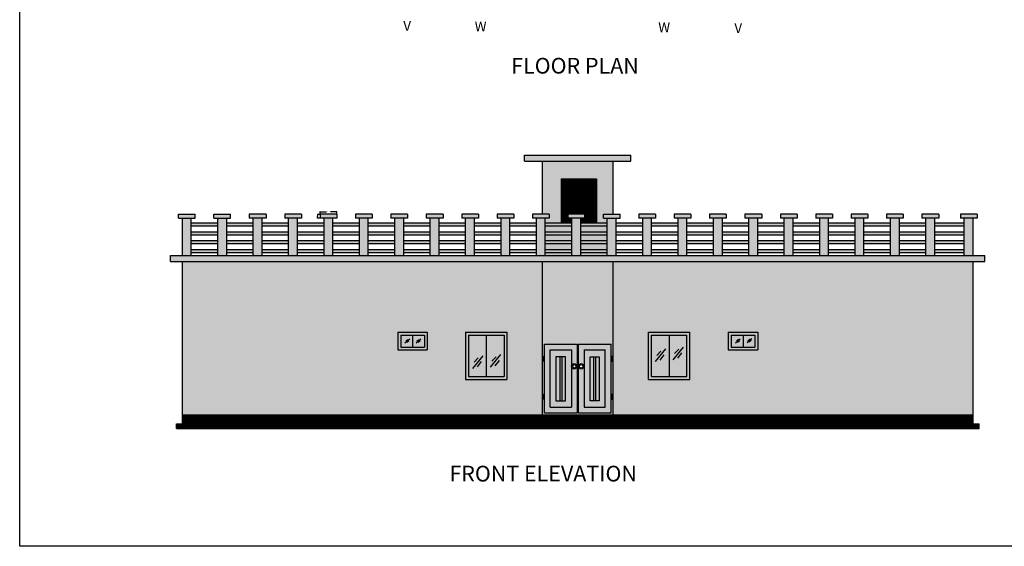
# Model space of a CAD drawing. Units: inches. Extents: x 9239 to 26065, y 6728 to 14611.
# Tile 1 of 12: x 9239 to 10240, y 6728 to 7264. Entities that reach past the tile are written whole.
import ezdxf

# ---------------------------------------------------------------- set-up
doc = ezdxf.new("R2010")
doc.units = ezdxf.units.IN
doc.header["$MEASUREMENT"] = 0
for name, color, linetype, lineweight in [('A-ANNO-DIMS', 2, 'Continuous', 18), ('A-ANNO-TEXT', 7, 'Continuous', 18), ('A-ELEV', 7, 'Continuous', 25), ('A-ELEV-PATT', 252, 'Continuous', 13), ('A-FLOR-STRS', 3, 'Continuous', 25)]:
    doc.layers.add(name, color=color, linetype=linetype, lineweight=lineweight)
doc.styles.get("Standard").update_dxf_attribs({"font": 'arial.ttf'})
doc.dimstyles.get("Standard").update_dxf_attribs({"dimtxt": 0.18, "dimasz": 0.18, "dimexe": 0.18, "dimexo": 0.0625, "dimgap": 0.09, "dimtad": 0, "dimtih": 1, "dimtoh": 1, "dimdec": 0, "dimzin": 0, "dimdsep": 46, "dimlunit": 3, "dimtxsty": 'Standard', "dimcen": 0.09, "dimadec": 0, "dimazin": 0, "dimtfac": 1, "dimtdec": 0, "dimtofl": 0, "dimtmove": 0, "dimatfit": 3, "dimfxl": 1, "dimtolj": 1, "dimtzin": 0, "dimarcsym": 0})

# ---------------------------------------------------------------- blocks, each defined once
blk = doc.blocks.new('ELEV-RAIL-POST')
for p, q in [((0, 4), (17, 4)), ((0, 0), (0, 4)), ((17, 0), (17, 4)), ((0, 0), (17, 0))]:
    blk.add_line(p, q)
blk = doc.blocks.new('*D48')
at = {"layer": 'A-ANNO-DIMS', "color": 0, "lineweight": -2, "transparency": 16777216}
for p, q in [((9544, 7065.9), (9544, 7068.6)), ((9544.2, 7068.4), (9550.6, 7068.4)), ((9560.9, 7068.4), (9554.5, 7068.4)), ((9561, 7065.9), (9561, 7068.6))]:
    blk.add_line(p, q, dxfattribs=at)
at = {"layer": 'A-ANNO-DIMS', "color": 0, "transparency": 16777216}
for points in [[(9544.2, 7068.4), (9544.2, 7068.4), (9544, 7068.4)], [(9560.9, 7068.4), (9560.9, 7068.4), (9561, 7068.4)]]:
    blk.add_solid(points, dxfattribs=at)
at = {"layer": 'Defpoints', "color": 0, "transparency": 16777216}
for p in [(9544, 7068.4), (9544, 7065.8), (9561, 7065.8)]:
    blk.add_point(p, dxfattribs=at)
at = {"layer": 'A-ANNO-DIMS', "color": 0, "transparency": 16777216, "insert": (9552.5, 7068.4), "char_height": 0.18, "attachment_point": 5}
blk.add_mtext('\\A1;PARAPET RAIL POST 1\'-5" TYP.', dxfattribs=at)
blk = doc.blocks.new('*D49')
at = {"layer": 'A-ANNO-DIMS', "color": 0, "lineweight": -2, "transparency": 16777216}
for p, q in [((9544, 7065.8), (9541.3, 7065.8)), ((9544, 7061.8), (9541.3, 7061.8)), ((9541.5, 7065.7), (9541.5, 7064)), ((9541.5, 7062), (9541.5, 7063.7))]:
    blk.add_line(p, q, dxfattribs=at)
at = {"layer": 'A-ANNO-DIMS', "color": 0, "transparency": 16777216}
for points in [[(9541.5, 7065.7), (9541.5, 7065.7), (9541.5, 7065.8)], [(9541.5, 7062), (9541.5, 7062), (9541.5, 7061.8)]]:
    blk.add_solid(points, dxfattribs=at)
at = {"layer": 'Defpoints', "color": 0, "transparency": 16777216}
for p in [(9541.5, 7061.8), (9544, 7065.8), (9544, 7061.8)]:
    blk.add_point(p, dxfattribs=at)
at = {"layer": 'A-ANNO-DIMS', "color": 0, "transparency": 16777216, "insert": (9541.5, 7063.8), "char_height": 0.18, "attachment_point": 5}
blk.add_mtext('\\A1;0\'-4" TYP.', dxfattribs=at)

msp = doc.modelspace()

# ---------------------------------------------------------------- hatches: boundary and pattern name
at = {"layer": 'A-ELEV-PATT'}
h = msp.add_hatch(color=256, dxfattribs=at)
h.dxf.hatch_style = 1
h.paths.add_polyline_path([(9752.05, 7125.85), (9752.05, 7119.85), (9860.05, 7119.85), (9860.05, 7125.85)])
h = msp.add_hatch(color=256, dxfattribs=at)
h.dxf.hatch_style = 1
h.paths.add_polyline_path([(9770.05, 7065.85), (9777.05, 7065.85), (9777.05, 7061.85), (9773.05, 7061.85), (9773.05, 7057.11), (9789.16, 7057.11), (9789.16, 7101.85), (9825.16, 7101.85), (9825.16, 7057.11), (9836.05, 7057.11), (9836.05, 7061.85), (9832.05, 7061.85), (9832.05, 7065.85), (9842.05, 7065.85), (9842.05, 7119.85), (9770.05, 7119.85)])
h.paths.add_polyline_path([(9800.05, 7048.11), (9800.05, 7054.11), (9773.05, 7054.11), (9773.05, 7048.11)])
h.paths.add_polyline_path([(9773.05, 7045.11), (9773.05, 7039.11), (9800.05, 7039.11), (9800.05, 7045.11)])
h.paths.add_polyline_path([(9773.05, 7036.11), (9773.05, 7030.11), (9800.05, 7030.11), (9800.05, 7036.11)])
h.paths.add_polyline_path([(9773.05, 7027.11), (9773.05, 7023.85), (9800.05, 7023.85), (9800.05, 7027.11)])
h.paths.add_polyline_path([(9836.05, 7023.85), (9836.05, 7027.11), (9809.05, 7027.11), (9809.05, 7023.85)])
h.paths.add_polyline_path([(9809.05, 7036.11), (9809.05, 7030.11), (9836.05, 7030.11), (9836.05, 7036.11)])
h.paths.add_polyline_path([(9809.05, 7045.11), (9809.05, 7039.11), (9836.05, 7039.11), (9836.05, 7045.11)])
h.paths.add_polyline_path([(9809.05, 7054.11), (9809.05, 7048.11), (9836.05, 7048.11), (9836.05, 7054.11)])
h = msp.add_hatch(dxfattribs=at)
h.set_pattern_fill('ANSI31', color=256)
h.set_pattern_definition([(45, (9789.16169, 7057.11151), (-0.08838835, 0.08838835), [])])
h.paths.add_polyline_path([(9825.16, 7101.85), (9789.16, 7101.85), (9789.16, 7057.11), (9794.16, 7057.11), (9794.16, 7096.85), (9820.16, 7096.85), (9820.16, 7057.11), (9825.16, 7057.11)])
h.paths.add_polyline_path([(9814.34, 7090.65), (9799.4, 7090.65), (9799.4, 7065.85), (9813.05, 7065.85), (9813.05, 7061.85), (9809.05, 7061.85), (9809.05, 7057.11), (9814.34, 7057.11)], flags=17)
h = msp.add_hatch(dxfattribs=at)
h.set_pattern_fill('ANSI31', color=256)
h.set_pattern_definition([(45, (9794.16169, 7057.11151), (-0.08838835, 0.08838835), [])])
h.paths.add_polyline_path([(9799.4, 7090.65), (9814.34, 7090.65), (9814.34, 7057.11), (9820.16, 7057.11), (9820.16, 7096.85), (9794.16, 7096.85), (9794.16, 7057.11), (9800.05, 7057.11), (9800.05, 7061.85), (9796.05, 7061.85), (9796.05, 7065.85), (9799.4, 7065.85)])
h = msp.add_hatch(color=256, dxfattribs=at)
h.dxf.hatch_style = 1
h.paths.add_polyline_path([(9392.05, 7023.85), (9392.05, 7017.85), (10220.05, 7017.85), (10220.05, 7023.85)])
h.paths.add_polyline_path([(9400.05, 7065.85), (9400.05, 7061.85), (9417.05, 7061.85), (9417.05, 7065.85)])
h.paths.add_polyline_path([(9453.05, 7061.85), (9453.05, 7065.85), (9436.05, 7065.85), (9436.05, 7061.85)])
h.paths.add_polyline_path([(9489.05, 7061.85), (9489.05, 7065.85), (9472.05, 7065.85), (9472.05, 7061.85)])
h.paths.add_polyline_path([(9525.05, 7065.85), (9508.05, 7065.85), (9508.05, 7061.85), (9525.05, 7061.85)])
h.paths.add_polyline_path([(9544.05, 7065.85), (9544.05, 7061.85), (9561.05, 7061.85), (9561.05, 7065.85)])
h.paths.add_polyline_path([(9597.05, 7061.85), (9597.05, 7065.85), (9580.05, 7065.85), (9580.05, 7061.85)])
h.paths.add_polyline_path([(9616.05, 7065.85), (9616.05, 7061.85), (9633.05, 7061.85), (9633.05, 7065.85)])
h.paths.add_polyline_path([(9652.05, 7065.85), (9652.05, 7061.85), (9669.05, 7061.85), (9669.05, 7065.85)])
h.paths.add_polyline_path([(9688.05, 7065.85), (9688.05, 7061.85), (9705.05, 7061.85), (9705.05, 7065.85)])
h.paths.add_polyline_path([(9741.05, 7061.85), (9741.05, 7065.85), (9724.05, 7065.85), (9724.05, 7061.85)])
h.paths.add_polyline_path([(9760.05, 7065.85), (9760.05, 7061.85), (9777.05, 7061.85), (9777.05, 7065.85)])
h.paths.add_polyline_path([(9796.05, 7065.85), (9796.05, 7061.85), (9813.05, 7061.85), (9813.05, 7065.85)])
h.paths.add_polyline_path([(9842.05, 7061.85), (9849.05, 7061.85), (9849.05, 7065.85), (9842.05, 7065.85), (9832.05, 7065.85), (9832.05, 7061.85)])
h.paths.add_polyline_path([(9885.05, 7061.85), (9885.05, 7065.85), (9868.05, 7065.85), (9868.05, 7061.85)])
h.paths.add_polyline_path([(9921.05, 7061.85), (9921.05, 7065.85), (9904.05, 7065.85), (9904.05, 7061.85)])
h.paths.add_polyline_path([(9940.05, 7065.85), (9940.05, 7061.85), (9957.05, 7061.85), (9957.05, 7065.85)])
h.paths.add_polyline_path([(9976.05, 7065.85), (9976.05, 7061.85), (9993.05, 7061.85), (9993.05, 7065.85)])
h.paths.add_polyline_path([(10029.05, 7065.85), (10012.05, 7065.85), (10012.05, 7061.85), (10029.05, 7061.85)])
h.paths.add_polyline_path([(10048.05, 7065.85), (10048.05, 7061.85), (10065.05, 7061.85), (10065.05, 7065.85)])
h.paths.add_polyline_path([(10101.05, 7061.85), (10101.05, 7065.85), (10084.05, 7065.85), (10084.05, 7061.85)])
h.paths.add_polyline_path([(10173.05, 7061.85), (10173.05, 7065.85), (10156.05, 7065.85), (10156.05, 7061.85)])
h.paths.add_polyline_path([(10137.05, 7061.85), (10137.05, 7065.85), (10120.05, 7065.85), (10120.05, 7061.85)])
h.paths.add_polyline_path([(10212.05, 7061.85), (10212.05, 7065.85), (10195.05, 7065.85), (10195.05, 7061.85)])
h = msp.add_hatch(color=256, dxfattribs=at)
h.dxf.hatch_style = 1
h.paths.add_polyline_path([(9404.05, 7023.85), (9413.05, 7023.85), (9413.05, 7061.85), (9404.05, 7061.85)])
h.paths.add_polyline_path([(9449.05, 7061.85), (9440.05, 7061.85), (9440.05, 7023.85), (9449.05, 7023.85)])
h.paths.add_polyline_path([(9476.05, 7023.85), (9485.05, 7023.85), (9485.05, 7061.85), (9476.05, 7061.85)])
h.paths.add_polyline_path([(9521.05, 7061.85), (9512.05, 7061.85), (9512.05, 7023.85), (9521.05, 7023.85)])
h.paths.add_polyline_path([(9557.05, 7061.85), (9548.05, 7061.85), (9548.05, 7023.85), (9557.05, 7023.85)])
h.paths.add_polyline_path([(9584.05, 7023.85), (9593.05, 7023.85), (9593.05, 7061.85), (9584.05, 7061.85)])
h.paths.add_polyline_path([(9620.05, 7023.85), (9629.05, 7023.85), (9629.05, 7061.85), (9620.05, 7061.85)])
h.paths.add_polyline_path([(9665.05, 7061.85), (9656.05, 7061.85), (9656.05, 7023.85), (9665.05, 7023.85)])
h.paths.add_polyline_path([(9692.05, 7023.85), (9701.05, 7023.85), (9701.05, 7061.85), (9692.05, 7061.85)])
h.paths.add_polyline_path([(9728.05, 7023.85), (9737.05, 7023.85), (9737.05, 7061.85), (9728.05, 7061.85)])
h.paths.add_polyline_path([(9773.05, 7061.85), (9764.05, 7061.85), (9764.05, 7023.85), (9773.05, 7023.85)])
h.paths.add_polyline_path([(9809.05, 7061.85), (9800.05, 7061.85), (9800.05, 7023.85), (9809.05, 7023.85)])
h.paths.add_polyline_path([(9845.05, 7061.85), (9842.05, 7061.85), (9836.05, 7061.85), (9836.05, 7023.85), (9845.05, 7023.85)])
h.paths.add_polyline_path([(9872.05, 7023.85), (9881.05, 7023.85), (9881.05, 7061.85), (9872.05, 7061.85)])
h.paths.add_polyline_path([(9917.05, 7061.85), (9908.05, 7061.85), (9908.05, 7023.85), (9917.05, 7023.85)])
h.paths.add_polyline_path([(9953.05, 7061.85), (9944.05, 7061.85), (9944.05, 7023.85), (9953.05, 7023.85)])
h.paths.add_polyline_path([(9980.05, 7023.85), (9989.05, 7023.85), (9989.05, 7061.85), (9980.05, 7061.85)])
h.paths.add_polyline_path([(10025.05, 7061.85), (10016.05, 7061.85), (10016.05, 7023.85), (10025.05, 7023.85)])
h.paths.add_polyline_path([(10061.05, 7061.85), (10052.05, 7061.85), (10052.05, 7023.85), (10061.05, 7023.85)])
h.paths.add_polyline_path([(10088.05, 7023.85), (10097.05, 7023.85), (10097.05, 7061.85), (10088.05, 7061.85)])
h.paths.add_polyline_path([(10133.05, 7061.85), (10124.05, 7061.85), (10124.05, 7023.85), (10133.05, 7023.85)])
h.paths.add_polyline_path([(10160.05, 7023.85), (10169.05, 7023.85), (10169.05, 7061.85), (10160.05, 7061.85)])
h.paths.add_polyline_path([(10208.05, 7061.85), (10199.05, 7061.85), (10199.05, 7023.85), (10208.05, 7023.85)])
h = msp.add_hatch(color=256, dxfattribs=at)
h.dxf.hatch_style = 1
h.paths.add_polyline_path([(9440.05, 7057.11), (9413.05, 7057.11), (9413.05, 7054.11), (9440.05, 7054.11)])
h.paths.add_polyline_path([(9440.05, 7048.11), (9413.05, 7048.11), (9413.05, 7045.11), (9440.05, 7045.11)])
h.paths.add_polyline_path([(9440.05, 7039.11), (9413.05, 7039.11), (9413.05, 7036.11), (9440.05, 7036.11)])
h.paths.add_polyline_path([(9440.05, 7030.11), (9413.05, 7030.11), (9413.05, 7027.11), (9440.05, 7027.11)])
h.paths.add_polyline_path([(9476.05, 7057.11), (9449.05, 7057.11), (9449.05, 7054.11), (9476.05, 7054.11)])
h.paths.add_polyline_path([(9476.05, 7048.11), (9449.05, 7048.11), (9449.05, 7045.11), (9476.05, 7045.11)])
h.paths.add_polyline_path([(9476.05, 7039.11), (9449.05, 7039.11), (9449.05, 7036.11), (9476.05, 7036.11)])
h.paths.add_polyline_path([(9476.05, 7030.11), (9449.05, 7030.11), (9449.05, 7027.11), (9476.05, 7027.11)])
h.paths.add_polyline_path([(9512.05, 7057.11), (9485.05, 7057.11), (9485.05, 7054.11), (9512.05, 7054.11)])
h.paths.add_polyline_path([(9512.05, 7048.11), (9485.05, 7048.11), (9485.05, 7045.11), (9512.05, 7045.11)])
h.paths.add_polyline_path([(9512.05, 7039.11), (9485.05, 7039.11), (9485.05, 7036.11), (9512.05, 7036.11)])
h.paths.add_polyline_path([(9512.05, 7030.11), (9485.05, 7030.11), (9485.05, 7027.11), (9512.05, 7027.11)])
h.paths.add_polyline_path([(9548.05, 7030.11), (9521.05, 7030.11), (9521.05, 7027.11), (9548.05, 7027.11)])
h.paths.add_polyline_path([(9548.05, 7039.11), (9521.05, 7039.11), (9521.05, 7036.11), (9548.05, 7036.11)])
h.paths.add_polyline_path([(9548.05, 7048.11), (9521.05, 7048.11), (9521.05, 7045.11), (9548.05, 7045.11)])
h.paths.add_polyline_path([(9548.05, 7057.11), (9521.05, 7057.11), (9521.05, 7054.11), (9548.05, 7054.11)])
h.paths.add_polyline_path([(9584.05, 7057.11), (9557.05, 7057.11), (9557.05, 7054.11), (9584.05, 7054.11)])
h.paths.add_polyline_path([(9620.05, 7057.11), (9593.05, 7057.11), (9593.05, 7054.11), (9620.05, 7054.11)])
h.paths.add_polyline_path([(9656.05, 7057.11), (9629.05, 7057.11), (9629.05, 7054.11), (9656.05, 7054.11)])
h.paths.add_polyline_path([(9656.05, 7048.11), (9629.05, 7048.11), (9629.05, 7045.11), (9656.05, 7045.11)])
h.paths.add_polyline_path([(9620.05, 7048.11), (9593.05, 7048.11), (9593.05, 7045.11), (9620.05, 7045.11)])
h.paths.add_polyline_path([(9584.05, 7048.11), (9557.05, 7048.11), (9557.05, 7045.11), (9584.05, 7045.11)])
h.paths.add_polyline_path([(9584.05, 7039.11), (9557.05, 7039.11), (9557.05, 7036.11), (9584.05, 7036.11)])
h.paths.add_polyline_path([(9620.05, 7039.11), (9593.05, 7039.11), (9593.05, 7036.11), (9620.05, 7036.11)])
h.paths.add_polyline_path([(9656.05, 7039.11), (9629.05, 7039.11), (9629.05, 7036.11), (9656.05, 7036.11)])
h.paths.add_polyline_path([(9656.05, 7030.11), (9629.05, 7030.11), (9629.05, 7027.11), (9656.05, 7027.11)])
h.paths.add_polyline_path([(9620.05, 7030.11), (9593.05, 7030.11), (9593.05, 7027.11), (9620.05, 7027.11)])
h.paths.add_polyline_path([(9584.05, 7030.11), (9557.05, 7030.11), (9557.05, 7027.11), (9584.05, 7027.11)])
h.paths.add_polyline_path([(9692.05, 7057.11), (9665.05, 7057.11), (9665.05, 7054.11), (9692.05, 7054.11)])
h.paths.add_polyline_path([(9728.05, 7057.11), (9701.05, 7057.11), (9701.05, 7054.11), (9728.05, 7054.11)])
h.paths.add_polyline_path([(9764.05, 7057.11), (9737.05, 7057.11), (9737.05, 7054.11), (9764.05, 7054.11)])
h.paths.add_polyline_path([(9764.05, 7048.11), (9737.05, 7048.11), (9737.05, 7045.11), (9764.05, 7045.11)])
h.paths.add_polyline_path([(9728.05, 7048.11), (9701.05, 7048.11), (9701.05, 7045.11), (9728.05, 7045.11)])
h.paths.add_polyline_path([(9692.05, 7048.11), (9665.05, 7048.11), (9665.05, 7045.11), (9692.05, 7045.11)])
h.paths.add_polyline_path([(9692.05, 7039.11), (9665.05, 7039.11), (9665.05, 7036.11), (9692.05, 7036.11)])
h.paths.add_polyline_path([(9728.05, 7039.11), (9701.05, 7039.11), (9701.05, 7036.11), (9728.05, 7036.11)])
h.paths.add_polyline_path([(9764.05, 7039.11), (9737.05, 7039.11), (9737.05, 7036.11), (9764.05, 7036.11)])
h.paths.add_polyline_path([(9692.05, 7030.11), (9665.05, 7030.11), (9665.05, 7027.11), (9692.05, 7027.11)])
h.paths.add_polyline_path([(9728.05, 7030.11), (9701.05, 7030.11), (9701.05, 7027.11), (9728.05, 7027.11)])
h.paths.add_polyline_path([(9764.05, 7030.11), (9737.05, 7030.11), (9737.05, 7027.11), (9764.05, 7027.11)])
h.paths.add_polyline_path([(9800.05, 7048.11), (9773.05, 7048.11), (9773.05, 7045.11), (9800.05, 7045.11)])
h.paths.add_polyline_path([(9800.05, 7057.11), (9773.05, 7057.11), (9773.05, 7054.11), (9800.05, 7054.11)])
h.paths.add_polyline_path([(9836.05, 7057.11), (9809.05, 7057.11), (9809.05, 7054.11), (9836.05, 7054.11)])
h.paths.add_polyline_path([(9836.05, 7048.11), (9809.05, 7048.11), (9809.05, 7045.11), (9836.05, 7045.11)])
h.paths.add_polyline_path([(9836.05, 7039.11), (9809.05, 7039.11), (9809.05, 7036.11), (9836.05, 7036.11)])
h.paths.add_polyline_path([(9800.05, 7039.11), (9773.05, 7039.11), (9773.05, 7036.11), (9800.05, 7036.11)])
h.paths.add_polyline_path([(9800.05, 7030.11), (9773.05, 7030.11), (9773.05, 7027.11), (9800.05, 7027.11)])
h.paths.add_polyline_path([(9836.05, 7030.11), (9809.05, 7030.11), (9809.05, 7027.11), (9836.05, 7027.11)])
h.paths.add_polyline_path([(9872.05, 7030.11), (9845.05, 7030.11), (9845.05, 7027.11), (9872.05, 7027.11)])
h.paths.add_polyline_path([(9872.05, 7039.11), (9845.05, 7039.11), (9845.05, 7036.11), (9872.05, 7036.11)])
h.paths.add_polyline_path([(9872.05, 7048.11), (9845.05, 7048.11), (9845.05, 7045.11), (9872.05, 7045.11)])
h.paths.add_polyline_path([(9872.05, 7057.11), (9845.05, 7057.11), (9845.05, 7054.11), (9872.05, 7054.11)])
h.paths.add_polyline_path([(9908.05, 7057.11), (9881.05, 7057.11), (9881.05, 7054.11), (9908.05, 7054.11)])
h.paths.add_polyline_path([(9908.05, 7048.11), (9881.05, 7048.11), (9881.05, 7045.11), (9908.05, 7045.11)])
h.paths.add_polyline_path([(9908.05, 7039.11), (9881.05, 7039.11), (9881.05, 7036.11), (9908.05, 7036.11)])
h.paths.add_polyline_path([(9908.05, 7030.11), (9881.05, 7030.11), (9881.05, 7027.11), (9908.05, 7027.11)])
h.paths.add_polyline_path([(9944.05, 7030.11), (9917.05, 7030.11), (9917.05, 7027.11), (9944.05, 7027.11)])
h.paths.add_polyline_path([(9944.05, 7039.11), (9917.05, 7039.11), (9917.05, 7036.11), (9944.05, 7036.11)])
h.paths.add_polyline_path([(9944.05, 7048.11), (9917.05, 7048.11), (9917.05, 7045.11), (9944.05, 7045.11)])
h.paths.add_polyline_path([(9944.05, 7057.11), (9917.05, 7057.11), (9917.05, 7054.11), (9944.05, 7054.11)])
h.paths.add_polyline_path([(9980.05, 7057.11), (9953.05, 7057.11), (9953.05, 7054.11), (9980.05, 7054.11)])
h.paths.add_polyline_path([(9980.05, 7048.11), (9953.05, 7048.11), (9953.05, 7045.11), (9980.05, 7045.11)])
h.paths.add_polyline_path([(9980.05, 7039.11), (9953.05, 7039.11), (9953.05, 7036.11), (9980.05, 7036.11)])
h.paths.add_polyline_path([(9980.05, 7030.11), (9953.05, 7030.11), (9953.05, 7027.11), (9980.05, 7027.11)])
h.paths.add_polyline_path([(10016.05, 7057.11), (9989.05, 7057.11), (9989.05, 7054.11), (10016.05, 7054.11)])
h.paths.add_polyline_path([(10016.05, 7048.11), (9989.05, 7048.11), (9989.05, 7045.11), (10016.05, 7045.11)])
h.paths.add_polyline_path([(10016.05, 7039.11), (9989.05, 7039.11), (9989.05, 7036.11), (10016.05, 7036.11)])
h.paths.add_polyline_path([(10052.05, 7057.11), (10025.05, 7057.11), (10025.05, 7054.11), (10052.05, 7054.11)])
h.paths.add_polyline_path([(10052.05, 7048.11), (10025.05, 7048.11), (10025.05, 7045.11), (10052.05, 7045.11)])
h.paths.add_polyline_path([(10052.05, 7039.11), (10025.05, 7039.11), (10025.05, 7036.11), (10052.05, 7036.11)])
h.paths.add_polyline_path([(10016.05, 7030.11), (9989.05, 7030.11), (9989.05, 7027.11), (10016.05, 7027.11)])
h.paths.add_polyline_path([(10052.05, 7030.11), (10025.05, 7030.11), (10025.05, 7027.11), (10052.05, 7027.11)])
h.paths.add_polyline_path([(10088.05, 7057.11), (10061.05, 7057.11), (10061.05, 7054.11), (10088.05, 7054.11)])
h.paths.add_polyline_path([(10088.05, 7048.11), (10061.05, 7048.11), (10061.05, 7045.11), (10088.05, 7045.11)])
h.paths.add_polyline_path([(10088.05, 7039.11), (10061.05, 7039.11), (10061.05, 7036.11), (10088.05, 7036.11)])
h.paths.add_polyline_path([(10088.05, 7030.11), (10061.05, 7030.11), (10061.05, 7027.11), (10088.05, 7027.11)])
h.paths.add_polyline_path([(10124.05, 7030.11), (10097.05, 7030.11), (10097.05, 7027.11), (10124.05, 7027.11)])
h.paths.add_polyline_path([(10124.05, 7039.11), (10097.05, 7039.11), (10097.05, 7036.11), (10124.05, 7036.11)])
h.paths.add_polyline_path([(10124.05, 7048.11), (10097.05, 7048.11), (10097.05, 7045.11), (10124.05, 7045.11)])
h.paths.add_polyline_path([(10124.05, 7057.11), (10097.05, 7057.11), (10097.05, 7054.11), (10124.05, 7054.11)])
h.paths.add_polyline_path([(10160.05, 7057.11), (10133.05, 7057.11), (10133.05, 7054.11), (10160.05, 7054.11)])
h.paths.add_polyline_path([(10199.05, 7057.11), (10169.05, 7057.11), (10169.05, 7054.11), (10199.05, 7054.11)])
h.paths.add_polyline_path([(10160.05, 7048.11), (10133.05, 7048.11), (10133.05, 7045.11), (10160.05, 7045.11)])
h.paths.add_polyline_path([(10199.05, 7048.11), (10169.05, 7048.11), (10169.05, 7045.11), (10199.05, 7045.11)])
h.paths.add_polyline_path([(10199.05, 7039.11), (10169.05, 7039.11), (10169.05, 7036.11), (10199.05, 7036.11)])
h.paths.add_polyline_path([(10160.05, 7039.11), (10133.05, 7039.11), (10133.05, 7036.11), (10160.05, 7036.11)])
h.paths.add_polyline_path([(10160.05, 7030.11), (10133.05, 7030.11), (10133.05, 7027.11), (10160.05, 7027.11)])
h.paths.add_polyline_path([(10199.05, 7030.11), (10169.05, 7030.11), (10169.05, 7027.11), (10199.05, 7027.11)])
h = msp.add_hatch(color=256, dxfattribs=at)
h.dxf.hatch_style = 1
h.paths.add_polyline_path([(9404.05, 7017.85), (9404.05, 6861.85), (9770.05, 6861.85), (9770.05, 7017.85)])
h.paths.add_polyline_path([(9623.05, 6945.85), (9653.05, 6945.85), (9653.05, 6927.85), (9623.05, 6927.85)], flags=16)
h.paths.add_polyline_path([(9626.05, 6942.85), (9650.05, 6942.85), (9650.05, 6930.85), (9626.05, 6930.85)], flags=0)
h.paths.add_polyline_path([(9692.05, 6945.85), (9734.05, 6945.85), (9734.05, 6897.85), (9692.05, 6897.85)], flags=16)
h.paths.add_polyline_path([(9695.05, 6942.85), (9731.05, 6942.85), (9731.05, 6900.85), (9695.05, 6900.85)], flags=0)
h.paths.add_polyline_path([(9842.05, 7017.85), (9842.05, 6861.85), (10208.05, 6861.85), (10208.05, 7017.85)])
h.paths.add_polyline_path([(9989.05, 6945.85), (9989.05, 6927.85), (9959.05, 6927.85), (9959.05, 6945.85)], flags=16)
h.paths.add_polyline_path([(9986.05, 6942.85), (9986.05, 6930.85), (9962.05, 6930.85), (9962.05, 6942.85)], flags=0)
h.paths.add_polyline_path([(9920.05, 6945.85), (9920.05, 6897.85), (9878.05, 6897.85), (9878.05, 6945.85)], flags=16)
h.paths.add_polyline_path([(9917.05, 6942.85), (9917.05, 6900.85), (9881.05, 6900.85), (9881.05, 6942.85)], flags=0)
h = msp.add_hatch(color=256, dxfattribs=at)
h.dxf.hatch_style = 1
h.paths.add_polyline_path([(9842.05, 7017.85), (9770.05, 7017.85), (9770.05, 6920.01), (9771.05, 6920.01), (9771.05, 6921.51), (9772.05, 6921.51), (9772.05, 6933.85), (9805.55, 6933.85), (9805.55, 6863.85), (9772.05, 6863.85), (9772.05, 6877.95), (9771.05, 6877.95), (9771.05, 6879.45), (9770.05, 6879.45), (9770.05, 6861.85), (9842.05, 6861.85), (9842.05, 6879.45), (9841.05, 6879.45), (9841.05, 6877.95), (9840.05, 6877.95), (9840.05, 6863.85), (9806.55, 6863.85), (9806.55, 6933.85), (9840.05, 6933.85), (9840.05, 6921.51), (9841.05, 6921.51), (9841.05, 6920.01), (9842.05, 6920.01)])
h.paths.add_polyline_path([(9772.05, 6916.51), (9771.05, 6916.51), (9771.05, 6918.01), (9770.05, 6918.01), (9770.05, 6881.45), (9771.05, 6881.45), (9771.05, 6882.95), (9772.05, 6882.95)], flags=17)
h.paths.add_polyline_path([(9842.05, 6918.01), (9841.05, 6918.01), (9841.05, 6916.51), (9840.05, 6916.51), (9840.05, 6882.95), (9841.05, 6882.95), (9841.05, 6881.45), (9842.05, 6881.45)], flags=17)
h.paths.add_polyline_path([(9827.64, 6920.86), (9824.18, 6920.86), (9824.18, 6876.3), (9827.64, 6876.3)], flags=17)
h.paths.add_polyline_path([(9822.18, 6920.86), (9818.72, 6920.86), (9818.72, 6876.3), (9822.18, 6876.3)], flags=17)
h.paths.add_polyline_path([(9793.31, 6921.25), (9789.75, 6921.25), (9789.75, 6875.72), (9793.31, 6875.72)], flags=17)
h.paths.add_polyline_path([(9787.75, 6921.25), (9784.19, 6921.25), (9784.19, 6875.72), (9787.75, 6875.72)], flags=17)
h = msp.add_hatch(color=256, dxfattribs=at)
h.dxf.hatch_style = 1
h.paths.add_polyline_path([(9623.05, 6945.85), (9623.05, 6927.85), (9653.05, 6927.85), (9653.05, 6945.85)])
h.paths.add_polyline_path([(9626.05, 6942.85), (9650.05, 6942.85), (9650.05, 6930.85), (9626.05, 6930.85)], flags=16)
h.paths.add_polyline_path([(9692.05, 6945.85), (9692.05, 6897.85), (9734.05, 6897.85), (9734.05, 6945.85)])
h.paths.add_polyline_path([(9695.05, 6942.85), (9731.05, 6942.85), (9731.05, 6900.85), (9695.05, 6900.85)], flags=16)
h.paths.add_polyline_path([(9878.05, 6897.85), (9920.05, 6897.85), (9920.05, 6945.85), (9878.05, 6945.85)])
h.paths.add_polyline_path([(9881.05, 6942.85), (9917.05, 6942.85), (9917.05, 6900.85), (9881.05, 6900.85)], flags=16)
h.paths.add_polyline_path([(9959.05, 6945.85), (9959.05, 6927.85), (9989.05, 6927.85), (9989.05, 6945.85)])
h.paths.add_polyline_path([(9962.05, 6942.85), (9986.05, 6942.85), (9986.05, 6930.85), (9962.05, 6930.85)], flags=16)
h = msp.add_hatch(color=256, dxfattribs=at)
h.dxf.hatch_style = 1
h.paths.add_polyline_path([(9638.05, 6942.85), (9626.05, 6942.85), (9626.05, 6930.85), (9638.05, 6930.85)])
h.paths.add_polyline_path([(9650.05, 6942.85), (9638.05, 6942.85), (9638.05, 6930.85), (9650.05, 6930.85)])
h.paths.add_polyline_path([(9713.05, 6942.85), (9695.05, 6942.85), (9695.05, 6900.85), (9713.05, 6900.85)])
h.paths.add_polyline_path([(9731.05, 6942.85), (9713.05, 6942.85), (9713.05, 6900.85), (9731.05, 6900.85)])
h.paths.add_polyline_path([(9899.05, 6942.85), (9881.05, 6942.85), (9881.05, 6900.85), (9899.05, 6900.85)])
h.paths.add_polyline_path([(9917.05, 6942.85), (9899.05, 6942.85), (9899.05, 6900.85), (9917.05, 6900.85)])
h.paths.add_polyline_path([(9974.05, 6942.85), (9962.05, 6942.85), (9962.05, 6930.85), (9974.05, 6930.85)])
h.paths.add_polyline_path([(9986.05, 6942.85), (9974.05, 6942.85), (9974.05, 6930.85), (9986.05, 6930.85)])
h = msp.add_hatch(color=256, dxfattribs=at)
h.dxf.hatch_style = 1
h.paths.add_polyline_path([(9772.05, 6921.51), (9771.05, 6921.51), (9771.05, 6916.51), (9772.05, 6916.51)])
h.paths.add_polyline_path([(9771.05, 6920.01), (9770.05, 6920.01), (9770.05, 6918.01), (9771.05, 6918.01)])
h.paths.add_polyline_path([(9772.05, 6882.95), (9771.05, 6882.95), (9771.05, 6877.95), (9772.05, 6877.95)])
h.paths.add_polyline_path([(9771.05, 6881.45), (9770.05, 6881.45), (9770.05, 6879.45), (9771.05, 6879.45)])
h.paths.add_polyline_path([(9841.05, 6882.95), (9840.05, 6882.95), (9840.05, 6877.95), (9841.05, 6877.95)])
h.paths.add_polyline_path([(9842.05, 6881.45), (9841.05, 6881.45), (9841.05, 6879.45), (9842.05, 6879.45)])
h.paths.add_polyline_path([(9841.05, 6921.51), (9840.05, 6921.51), (9840.05, 6916.51), (9841.05, 6916.51)])
h.paths.add_polyline_path([(9842.05, 6920.01), (9841.05, 6920.01), (9841.05, 6918.01), (9842.05, 6918.01)])
h.paths.add_polyline_path([(9840.05, 6933.85), (9806.55, 6933.85), (9806.55, 6863.85), (9840.05, 6863.85)])
h.paths.add_polyline_path([(9834.05, 6869.85), (9812.55, 6869.85), (9812.55, 6927.85), (9834.05, 6927.85)], flags=16)
h.paths.add_polyline_path([(9827.64, 6876.3), (9818.72, 6876.3), (9818.72, 6920.86), (9827.64, 6920.86)], flags=0)
h.paths.add_polyline_path([(9812.34, 6911.29, -1), (9806.76, 6911.29, -1)], flags=16)
h.paths.add_polyline_path([(9811.34, 6911.29, -1), (9807.76, 6911.29, -1)], flags=0)
h.paths.add_polyline_path([(9805.55, 6933.85), (9772.05, 6933.85), (9772.05, 6863.85), (9805.55, 6863.85)])
h.paths.add_polyline_path([(9799.55, 6869.85), (9778.05, 6869.85), (9778.05, 6927.85), (9799.55, 6927.85)], flags=16)
h.paths.add_polyline_path([(9793.31, 6875.72), (9784.19, 6875.72), (9784.19, 6921.25), (9793.31, 6921.25)], flags=0)
h.paths.add_polyline_path([(9799.69, 6911.29, -1), (9805.27, 6911.29, -1)], flags=16)
h.paths.add_polyline_path([(9800.69, 6911.29, -1), (9804.27, 6911.29, -1)], flags=0)
h.paths.add_polyline_path([(9789.75, 6921.25), (9787.75, 6921.25), (9787.75, 6875.72), (9789.75, 6875.72)], flags=0)
h = msp.add_hatch(color=256, dxfattribs=at)
h.dxf.hatch_style = 1
h.paths.add_polyline_path([(9778.05, 6869.85), (9799.55, 6869.85), (9799.55, 6927.85), (9778.05, 6927.85)])
h.paths.add_polyline_path([(9784.19, 6921.25), (9793.31, 6921.25), (9793.31, 6875.72), (9784.19, 6875.72)], flags=16)
h.paths.add_polyline_path([(9812.55, 6869.85), (9834.05, 6869.85), (9834.05, 6927.85), (9812.55, 6927.85)])
h.paths.add_polyline_path([(9818.72, 6920.86), (9827.64, 6920.86), (9827.64, 6876.3), (9818.72, 6876.3)], flags=16)
h = msp.add_hatch(color=256, dxfattribs=at)
h.dxf.hatch_style = 1
h.paths.add_polyline_path([(9787.75, 6875.72), (9789.75, 6875.72), (9789.75, 6921.25), (9787.75, 6921.25)])
h.paths.add_polyline_path([(9824.18, 6920.86), (9822.18, 6920.86), (9822.18, 6876.3), (9824.18, 6876.3)])
h = msp.add_hatch(dxfattribs=at)
h.set_pattern_fill('ANSI31', color=256)
h.set_pattern_definition([(45, (9404.04947, 6852.84587), (-0.088388348, 0.088388348), [])])
h.paths.add_polyline_path([(10208.05, 6852.85), (10208.05, 6861.85), (9404.05, 6861.85), (9404.05, 6852.85)])
h = msp.add_hatch(dxfattribs=at)
h.set_pattern_fill('ANSI31', color=256)
h.set_pattern_definition([(45, (9398.04947, 6847.84587), (-0.088388348, 0.088388348), [])])
h.paths.add_polyline_path([(9398.05, 6852.85), (9398.05, 6847.85), (10214.05, 6847.85), (10214.05, 6852.85)])

# ---------------------------------------------------------------- linework, layer by layer
at = {"layer": 'A-ELEV'}
for p, q in [((9752.05, 7125.85), (9860.05, 7125.85)), ((9752.05, 7119.85), (9752.05, 7125.85)), ((9752.05, 7119.85), (9860.05, 7119.85)), ((9770.05, 7065.85), (9770.05, 7119.85)), ((9842.05, 7065.85), (9842.05, 7119.85)), ((9860.05, 7119.85), (9860.05, 7125.85)), ((9789.16, 7101.85), (9825.16, 7101.85)), ((9789.16, 7101.85), (9789.16, 7057.11)), ((9825.16, 7101.85), (9825.16, 7057.11)), ((9794.16, 7096.85), (9794.16, 7057.11)), ((9794.16, 7096.85), (9820.16, 7096.85)), ((9820.16, 7096.85), (9820.16, 7057.11)), ((9404.05, 7023.85), (9404.05, 7061.85)), ((9413.05, 7023.85), (9413.05, 7061.85)), ((9440.05, 7023.85), (9440.05, 7061.85)), ((9449.05, 7023.85), (9449.05, 7061.85)), ((9476.05, 7023.85), (9476.05, 7061.85)), ((9485.05, 7023.85), (9485.05, 7061.85)), ((9512.05, 7023.85), (9512.05, 7061.85)), ((9521.05, 7023.85), (9521.05, 7061.85)), ((9548.05, 7023.85), (9548.05, 7061.85)), ((9557.05, 7023.85), (9557.05, 7061.85)), ((9584.05, 7023.85), (9584.05, 7061.85)), ((9593.05, 7023.85), (9593.05, 7061.85)), ((9620.05, 7023.85), (9620.05, 7061.85)), ((9629.05, 7023.85), (9629.05, 7061.85)), ((9656.05, 7023.85), (9656.05, 7061.85)), ((9665.05, 7023.85), (9665.05, 7061.85)), ((9692.05, 7023.85), (9692.05, 7061.85)), ((9701.05, 7023.85), (9701.05, 7061.85)), ((9728.05, 7023.85), (9728.05, 7061.85)), ((9737.05, 7023.85), (9737.05, 7061.85)), ((9764.05, 7023.85), (9764.05, 7061.85)), ((9773.05, 7023.85), (9773.05, 7061.85)), ((9800.05, 7023.85), (9800.05, 7061.85)), ((9809.05, 7023.85), (9809.05, 7061.85)), ((9832.05, 7061.85), (9832.05, 7065.85)), ((9832.05, 7065.85), (9842.05, 7065.85)), ((9832.05, 7061.85), (9842.05, 7061.85)), ((9836.05, 7023.85), (9836.05, 7061.85)), ((9842.05, 7065.85), (9849.05, 7065.85)), ((9842.05, 7061.85), (9849.05, 7061.85)), ((9845.05, 7023.85), (9845.05, 7061.85)), ((9849.05, 7061.85), (9849.05, 7065.85)), ((9872.05, 7023.85), (9872.05, 7061.85)), ((9881.05, 7023.85), (9881.05, 7061.85)), ((9908.05, 7023.85), (9908.05, 7061.85)), ((9917.05, 7023.85), (9917.05, 7061.85)), ((9944.05, 7023.85), (9944.05, 7061.85)), ((9953.05, 7023.85), (9953.05, 7061.85)), ((9980.05, 7023.85), (9980.05, 7061.85)), ((9989.05, 7023.85), (9989.05, 7061.85)), ((10016.05, 7023.85), (10016.05, 7061.85)), ((10025.05, 7023.85), (10025.05, 7061.85)), ((10052.05, 7023.85), (10052.05, 7061.85)), ((10061.05, 7023.85), (10061.05, 7061.85)), ((10088.05, 7023.85), (10088.05, 7061.85)), ((10097.05, 7023.85), (10097.05, 7061.85)), ((10124.05, 7023.85), (10124.05, 7061.85)), ((10133.05, 7023.85), (10133.05, 7061.85)), ((10160.05, 7023.85), (10160.05, 7061.85)), ((10169.05, 7023.85), (10169.05, 7061.85)), ((10199.05, 7023.85), (10199.05, 7061.85)), ((10208.05, 7023.85), (10208.05, 7061.85)), ((9413.05, 7057.11), (9440.05, 7057.11)), ((9413.05, 7054.11), (9440.05, 7054.11)), ((9413.05, 7048.11), (9440.05, 7048.11)), ((9449.05, 7057.11), (9476.05, 7057.11)), ((9449.05, 7054.11), (9476.05, 7054.11)), ((9449.05, 7048.11), (9476.05, 7048.11)), ((9485.05, 7057.11), (9512.05, 7057.11)), ((9485.05, 7054.11), (9512.05, 7054.11)), ((9485.05, 7048.11), (9512.05, 7048.11)), ((9521.05, 7057.11), (9548.05, 7057.11)), ((9521.05, 7054.11), (9548.05, 7054.11)), ((9521.05, 7048.11), (9548.05, 7048.11)), ((9557.05, 7057.11), (9584.05, 7057.11)), ((9557.05, 7054.11), (9584.05, 7054.11)), ((9557.05, 7048.11), (9584.05, 7048.11)), ((9593.05, 7057.11), (9620.05, 7057.11)), ((9593.05, 7054.11), (9620.05, 7054.11)), ((9593.05, 7048.11), (9620.05, 7048.11)), ((9629.05, 7057.11), (9656.05, 7057.11)), ((9629.05, 7054.11), (9656.05, 7054.11)), ((9629.05, 7048.11), (9656.05, 7048.11)), ((9665.05, 7057.11), (9692.05, 7057.11)), ((9665.05, 7054.11), (9692.05, 7054.11)), ((9665.05, 7048.11), (9692.05, 7048.11)), ((9701.05, 7057.11), (9728.05, 7057.11)), ((9701.05, 7054.11), (9728.05, 7054.11)), ((9701.05, 7048.11), (9728.05, 7048.11)), ((9737.05, 7057.11), (9764.05, 7057.11)), ((9737.05, 7054.11), (9764.05, 7054.11)), ((9737.05, 7048.11), (9764.05, 7048.11)), ((9773.05, 7057.11), (9800.05, 7057.11)), ((9773.05, 7054.11), (9800.05, 7054.11)), ((9773.05, 7048.11), (9800.05, 7048.11)), ((9809.05, 7057.11), (9836.05, 7057.11)), ((9809.05, 7054.11), (9836.05, 7054.11)), ((9809.05, 7048.11), (9836.05, 7048.11)), ((9845.05, 7057.11), (9872.05, 7057.11)), ((9845.05, 7054.11), (9872.05, 7054.11)), ((9845.05, 7048.11), (9872.05, 7048.11)), ((9881.05, 7057.11), (9908.05, 7057.11)), ((9881.05, 7054.11), (9908.05, 7054.11)), ((9881.05, 7048.11), (9908.05, 7048.11)), ((9917.05, 7057.11), (9944.05, 7057.11)), ((9917.05, 7054.11), (9944.05, 7054.11)), ((9917.05, 7048.11), (9944.05, 7048.11)), ((9953.05, 7057.11), (9980.05, 7057.11)), ((9953.05, 7054.11), (9980.05, 7054.11)), ((9953.05, 7048.11), (9980.05, 7048.11)), ((9989.05, 7057.11), (10016.05, 7057.11)), ((9989.05, 7054.11), (10016.05, 7054.11)), ((9989.05, 7048.11), (10016.05, 7048.11)), ((10025.05, 7057.11), (10052.05, 7057.11)), ((10025.05, 7054.11), (10052.05, 7054.11)), ((10025.05, 7048.11), (10052.05, 7048.11)), ((10061.05, 7057.11), (10088.05, 7057.11)), ((10061.05, 7054.11), (10088.05, 7054.11)), ((10061.05, 7048.11), (10088.05, 7048.11)), ((10097.05, 7057.11), (10124.05, 7057.11)), ((10097.05, 7054.11), (10124.05, 7054.11)), ((10097.05, 7048.11), (10124.05, 7048.11)), ((10133.05, 7057.11), (10160.05, 7057.11)), ((10133.05, 7054.11), (10160.05, 7054.11)), ((10133.05, 7048.11), (10160.05, 7048.11)), ((10169.05, 7057.11), (10199.05, 7057.11)), ((10169.05, 7054.11), (10199.05, 7054.11)), ((10169.05, 7048.11), (10199.05, 7048.11)), ((9413.05, 7045.11), (9440.05, 7045.11)), ((9413.05, 7039.11), (9440.05, 7039.11)), ((9449.05, 7045.11), (9476.05, 7045.11)), ((9449.05, 7039.11), (9476.05, 7039.11)), ((9485.05, 7045.11), (9512.05, 7045.11)), ((9485.05, 7039.11), (9512.05, 7039.11)), ((9521.05, 7045.11), (9548.05, 7045.11)), ((9521.05, 7039.11), (9548.05, 7039.11)), ((9557.05, 7045.11), (9584.05, 7045.11)), ((9557.05, 7039.11), (9584.05, 7039.11)), ((9593.05, 7045.11), (9620.05, 7045.11)), ((9593.05, 7039.11), (9620.05, 7039.11)), ((9629.05, 7045.11), (9656.05, 7045.11)), ((9629.05, 7039.11), (9656.05, 7039.11)), ((9665.05, 7045.11), (9692.05, 7045.11)), ((9665.05, 7039.11), (9692.05, 7039.11)), ((9701.05, 7045.11), (9728.05, 7045.11)), ((9701.05, 7039.11), (9728.05, 7039.11)), ((9737.05, 7045.11), (9764.05, 7045.11)), ((9737.05, 7039.11), (9764.05, 7039.11)), ((9773.05, 7045.11), (9800.05, 7045.11)), ((9773.05, 7039.11), (9800.05, 7039.11)), ((9809.05, 7045.11), (9836.05, 7045.11)), ((9809.05, 7039.11), (9836.05, 7039.11)), ((9845.05, 7045.11), (9872.05, 7045.11)), ((9845.05, 7039.11), (9872.05, 7039.11)), ((9881.05, 7045.11), (9908.05, 7045.11)), ((9881.05, 7039.11), (9908.05, 7039.11)), ((9917.05, 7045.11), (9944.05, 7045.11)), ((9917.05, 7039.11), (9944.05, 7039.11)), ((9953.05, 7045.11), (9980.05, 7045.11)), ((9953.05, 7039.11), (9980.05, 7039.11)), ((9989.05, 7045.11), (10016.05, 7045.11)), ((9989.05, 7039.11), (10016.05, 7039.11)), ((10025.05, 7045.11), (10052.05, 7045.11)), ((10025.05, 7039.11), (10052.05, 7039.11)), ((10061.05, 7045.11), (10088.05, 7045.11)), ((10061.05, 7039.11), (10088.05, 7039.11)), ((10097.05, 7045.11), (10124.05, 7045.11)), ((10097.05, 7039.11), (10124.05, 7039.11)), ((10133.05, 7045.11), (10160.05, 7045.11)), ((10133.05, 7039.11), (10160.05, 7039.11)), ((10169.05, 7045.11), (10199.05, 7045.11)), ((10169.05, 7039.11), (10199.05, 7039.11)), ((9413.05, 7036.11), (9440.05, 7036.11)), ((9413.05, 7030.11), (9440.05, 7030.11)), ((9449.05, 7036.11), (9476.05, 7036.11)), ((9449.05, 7030.11), (9476.05, 7030.11)), ((9485.05, 7036.11), (9512.05, 7036.11)), ((9485.05, 7030.11), (9512.05, 7030.11)), ((9521.05, 7036.11), (9548.05, 7036.11)), ((9521.05, 7030.11), (9548.05, 7030.11)), ((9557.05, 7036.11), (9584.05, 7036.11)), ((9557.05, 7030.11), (9584.05, 7030.11)), ((9593.05, 7036.11), (9620.05, 7036.11)), ((9593.05, 7030.11), (9620.05, 7030.11)), ((9629.05, 7036.11), (9656.05, 7036.11)), ((9629.05, 7030.11), (9656.05, 7030.11)), ((9665.05, 7036.11), (9692.05, 7036.11)), ((9665.05, 7030.11), (9692.05, 7030.11)), ((9701.05, 7036.11), (9728.05, 7036.11)), ((9701.05, 7030.11), (9728.05, 7030.11)), ((9737.05, 7036.11), (9764.05, 7036.11)), ((9737.05, 7030.11), (9764.05, 7030.11)), ((9773.05, 7036.11), (9800.05, 7036.11)), ((9773.05, 7030.11), (9800.05, 7030.11)), ((9809.05, 7036.11), (9836.05, 7036.11)), ((9809.05, 7030.11), (9836.05, 7030.11)), ((9845.05, 7036.11), (9872.05, 7036.11)), ((9845.05, 7030.11), (9872.05, 7030.11)), ((9881.05, 7036.11), (9908.05, 7036.11)), ((9881.05, 7030.11), (9908.05, 7030.11)), ((9917.05, 7036.11), (9944.05, 7036.11)), ((9917.05, 7030.11), (9944.05, 7030.11)), ((9953.05, 7036.11), (9980.05, 7036.11)), ((9953.05, 7030.11), (9980.05, 7030.11)), ((9989.05, 7036.11), (10016.05, 7036.11)), ((9989.05, 7030.11), (10016.05, 7030.11)), ((10025.05, 7036.11), (10052.05, 7036.11)), ((10025.05, 7030.11), (10052.05, 7030.11)), ((10061.05, 7036.11), (10088.05, 7036.11)), ((10061.05, 7030.11), (10088.05, 7030.11)), ((10097.05, 7036.11), (10124.05, 7036.11)), ((10097.05, 7030.11), (10124.05, 7030.11)), ((10133.05, 7036.11), (10160.05, 7036.11)), ((10133.05, 7030.11), (10160.05, 7030.11)), ((10169.05, 7036.11), (10199.05, 7036.11)), ((10169.05, 7030.11), (10199.05, 7030.11)), ((9392.05, 7023.85), (10220.05, 7023.85)), ((9392.05, 7017.85), (9392.05, 7023.85)), ((9404.05, 7023.85), (9404.05, 7023.85)), ((9413.05, 7027.11), (9440.05, 7027.11)), ((9449.05, 7027.11), (9476.05, 7027.11)), ((9485.05, 7027.11), (9512.05, 7027.11)), ((9521.05, 7027.11), (9548.05, 7027.11)), ((9557.05, 7027.11), (9584.05, 7027.11)), ((9593.05, 7027.11), (9620.05, 7027.11)), ((9629.05, 7027.11), (9656.05, 7027.11)), ((9665.05, 7027.11), (9692.05, 7027.11)), ((9701.05, 7027.11), (9728.05, 7027.11)), ((9737.05, 7027.11), (9764.05, 7027.11)), ((9773.05, 7027.11), (9800.05, 7027.11)), ((9809.05, 7027.11), (9836.05, 7027.11)), ((9845.05, 7027.11), (9872.05, 7027.11)), ((9881.05, 7027.11), (9908.05, 7027.11)), ((9917.05, 7027.11), (9944.05, 7027.11)), ((9953.05, 7027.11), (9980.05, 7027.11)), ((9989.05, 7027.11), (10016.05, 7027.11)), ((10025.05, 7027.11), (10052.05, 7027.11)), ((10061.05, 7027.11), (10088.05, 7027.11)), ((10097.05, 7027.11), (10124.05, 7027.11)), ((10133.05, 7027.11), (10160.05, 7027.11)), ((10169.05, 7027.11), (10199.05, 7027.11)), ((10208.05, 7023.85), (10208.05, 7023.85)), ((10220.05, 7017.85), (10220.05, 7023.85)), ((9392.05, 7017.85), (10220.05, 7017.85)), ((9404.05, 6852.85), (9404.05, 7017.85)), ((9770.05, 6861.85), (9770.05, 7017.85)), ((9842.05, 6861.85), (9842.05, 7017.85)), ((10208.05, 6852.85), (10208.05, 7017.85)), ((9623.05, 6945.85), (9623.05, 6927.85)), ((9623.05, 6945.85), (9653.05, 6945.85)), ((9626.05, 6942.85), (9626.05, 6930.85)), ((9626.05, 6942.85), (9650.05, 6942.85)), ((9630.28, 6935.12), (9635.19, 6939.05)), ((9631.16, 6936.77), (9633.39, 6938.66)), ((9638.05, 6942.85), (9638.05, 6930.85)), ((9641.67, 6935.14), (9646.57, 6939.07)), ((9642.54, 6936.79), (9644.77, 6938.68)), ((9650.05, 6942.85), (9650.05, 6930.85)), ((9653.05, 6945.85), (9653.05, 6927.85)), ((9692.05, 6945.85), (9692.05, 6897.85)), ((9692.05, 6945.85), (9734.05, 6945.85)), ((9695.05, 6942.85), (9695.05, 6900.85)), ((9695.05, 6942.85), (9731.05, 6942.85)), ((9713.05, 6942.85), (9713.05, 6900.85)), ((9731.05, 6942.85), (9731.05, 6900.85)), ((9734.05, 6945.85), (9734.05, 6897.85)), ((9878.05, 6897.85), (9878.05, 6945.85)), ((9878.05, 6945.85), (9920.05, 6945.85)), ((9881.05, 6900.85), (9881.05, 6942.85)), ((9881.05, 6942.85), (9917.05, 6942.85)), ((9899.05, 6942.85), (9899.05, 6900.85)), ((9917.05, 6900.85), (9917.05, 6942.85)), ((9920.05, 6897.85), (9920.05, 6945.85)), ((9959.05, 6945.85), (9959.05, 6927.85)), ((9959.05, 6945.85), (9989.05, 6945.85)), ((9962.05, 6942.85), (9962.05, 6930.85)), ((9962.05, 6942.85), (9986.05, 6942.85)), ((9966.42, 6935.23), (9971.32, 6939.15)), ((9967.3, 6936.87), (9969.53, 6938.77)), ((9974.05, 6942.85), (9974.05, 6930.85)), ((9978.12, 6935.62), (9983.02, 6939.55)), ((9978.99, 6937.27), (9981.23, 6939.16)), ((9986.05, 6942.85), (9986.05, 6930.85)), ((9989.05, 6945.85), (9989.05, 6927.85)), ((9626.05, 6930.85), (9650.05, 6930.85)), ((9632.22, 6935.8), (9634.41, 6937.45)), ((9643.61, 6935.82), (9645.79, 6937.47)), ((9772.05, 6933.85), (9805.55, 6933.85)), ((9772.05, 6863.85), (9772.05, 6933.85)), ((9805.55, 6933.85), (9805.55, 6863.85)), ((9806.55, 6933.85), (9806.55, 6863.85)), ((9806.55, 6933.85), (9840.05, 6933.85)), ((9840.05, 6863.85), (9840.05, 6933.85)), ((9884.96, 6916), (9895.42, 6928.88)), ((9903.14, 6917.96), (9913.6, 6930.83)), ((9904.48, 6924.15), (9908.73, 6928.64)), ((9962.05, 6930.85), (9986.05, 6930.85)), ((9968.36, 6935.9), (9970.55, 6937.55)), ((9980.06, 6936.3), (9982.25, 6937.95)), ((9623.05, 6927.85), (9653.05, 6927.85)), ((9699.34, 6909.15), (9709.8, 6922.03)), ((9700.67, 6915.35), (9704.93, 6919.84)), ((9717.46, 6910.25), (9727.91, 6923.12)), ((9718.79, 6916.44), (9723.05, 6920.94)), ((9770.05, 6920.01), (9771.05, 6920.01)), ((9770.05, 6918.01), (9771.05, 6918.01)), ((9771.05, 6921.51), (9772.05, 6921.51)), ((9771.05, 6921.51), (9771.05, 6916.51)), ((9778.05, 6927.85), (9799.55, 6927.85)), ((9778.05, 6869.85), (9778.05, 6927.85)), ((9787.75, 6921.25), (9787.75, 6875.72)), ((9789.75, 6921.25), (9789.75, 6875.72)), ((9799.55, 6927.85), (9799.55, 6869.85)), ((9812.55, 6927.85), (9834.05, 6927.85)), ((9812.55, 6927.85), (9812.55, 6869.85)), ((9822.18, 6920.86), (9822.18, 6876.3)), ((9824.18, 6920.86), (9824.18, 6876.3)), ((9834.05, 6869.85), (9834.05, 6927.85)), ((9840.05, 6921.51), (9841.05, 6921.51)), ((9841.05, 6921.51), (9841.05, 6916.51)), ((9841.05, 6920.01), (9842.05, 6920.01)), ((9841.05, 6918.01), (9842.05, 6918.01)), ((9886.29, 6922.2), (9890.55, 6926.69)), ((9889.7, 6917.46), (9893.83, 6922.93)), ((9907.88, 6919.41), (9912.02, 6924.88)), ((9959.05, 6927.85), (9989.05, 6927.85)), ((9704.08, 6910.61), (9708.21, 6916.08)), ((9722.2, 6911.71), (9726.33, 6917.17)), ((9771.05, 6916.51), (9772.05, 6916.51)), ((9840.05, 6916.51), (9841.05, 6916.51)), ((9695.05, 6900.85), (9731.05, 6900.85)), ((9881.05, 6900.85), (9917.05, 6900.85)), ((9692.05, 6897.85), (9734.05, 6897.85)), ((9878.05, 6897.85), (9920.05, 6897.85)), ((9770.05, 6881.45), (9771.05, 6881.45)), ((9770.05, 6879.45), (9771.05, 6879.45)), ((9771.05, 6882.95), (9772.05, 6882.95)), ((9771.05, 6882.95), (9771.05, 6877.95)), ((9771.05, 6877.95), (9772.05, 6877.95)), ((9840.05, 6882.95), (9841.05, 6882.95)), ((9840.05, 6877.95), (9841.05, 6877.95)), ((9841.05, 6882.95), (9841.05, 6877.95)), ((9841.05, 6881.45), (9842.05, 6881.45)), ((9841.05, 6879.45), (9842.05, 6879.45)), ((9778.05, 6869.85), (9799.55, 6869.85)), ((9812.55, 6869.85), (9834.05, 6869.85)), ((9404.05, 6861.85), (10208.05, 6861.85)), ((9772.05, 6863.85), (9805.55, 6863.85)), ((9806.55, 6863.85), (9840.05, 6863.85)), ((9398.05, 6852.85), (10214.05, 6852.85)), ((9398.05, 6847.85), (9398.05, 6852.85)), ((10214.05, 6847.85), (10214.05, 6852.85)), ((9398.05, 6847.85), (10214.05, 6847.85))]:
    msp.add_line(p, q, dxfattribs=at)
msp.add_lwpolyline([(9799.4, 7065.85), (9799.4, 7090.65), (9814.34, 7090.65), (9814.34, 7057.11)], dxfattribs=at)
for points in [[(9784.19, 6921.25), (9793.31, 6921.25), (9793.31, 6875.72), (9784.19, 6875.72)], [(9818.72, 6920.86), (9827.64, 6920.86), (9827.64, 6876.3), (9818.72, 6876.3)]]:
    msp.add_lwpolyline(points, close=True, dxfattribs=at)
for centre, radius in [((9802.48, 6911.29), 2.79), ((9802.48, 6911.29), 1.79), ((9809.55, 6911.29), 2.79), ((9809.55, 6911.29), 1.79)]:
    msp.add_circle(centre, radius, dxfattribs=at)
at = {"layer": 'A-FLOR-STRS'}
msp.add_lwpolyline([(9238.6, 7933.95), (11208.24, 7933.95), (11208.24, 6728.19), (9238.6, 6728.19)], close=True, dxfattribs=at)

# ---------------------------------------------------------------- block references
at = {"layer": 'A-ELEV'}
for p in [(9400.05, 7061.85), (9436.05, 7061.85)]:
    msp.add_blockref('ELEV-RAIL-POST', p, dxfattribs=at)
at = {"layer": 'A-ELEV', "rotation": 180}
for p in [(9489.05, 7065.85), (9525.05, 7065.85), (9561.05, 7065.85), (9597.05, 7065.85), (9633.05, 7065.85), (9669.05, 7065.85), (9705.05, 7065.85), (9741.05, 7065.85), (9777.05, 7065.85), (9813.05, 7065.85), (9885.05, 7065.85), (9921.05, 7065.85), (9957.05, 7065.85), (9993.05, 7065.85), (10029.05, 7065.85), (10065.05, 7065.85), (10101.05, 7065.85), (10137.05, 7065.85), (10173.05, 7065.85), (10212.05, 7065.85)]:
    msp.add_blockref('ELEV-RAIL-POST', p, dxfattribs=at)

# ---------------------------------------------------------------- texts
at = {"layer": 'A-ANNO-TEXT', "attachment_point": 1}
for s, width, insert, char_height in [('V', 325.9721, (9628.64, 7262.48), 10), ('W', 325.9721, (9701.28, 7261.92), 10), ('W', 325.9721, (9887.94, 7260.95), 10), ('V', 325.9721, (9965.27, 7260.22), 10), ('FLOOR PLAN', 834.9824, (9738.34, 7224.97), 16), ('FRONT ELEVATION', 797.6691, (9675.52, 6810.15), 16)]:
    msp.add_mtext_dynamic_manual_height_columns(s, width=width, gutter_width=1, heights=[0], dxfattribs=dict(at, insert=insert, char_height=char_height))

# ---------------------------------------------------------------- dimensions: what is measured, and where the dimension line sits
at = {"layer": 'A-ANNO-DIMS'}
for base, p1, p2, angle, text, picture, middle in [((9544.05, 7068.4), (9561.05, 7065.85), (9544.05, 7065.85), 180, 'PARAPET RAIL POST <> TYP.', '*D48', (9552.55, 7068.4)), ((9541.5, 7061.85), (9544.05, 7065.85), (9544.05, 7061.85), 270, '<> TYP.', '*D49', (9541.5, 7063.85))]:
    dim = msp.add_linear_dim(base=base, p1=p1, p2=p2, angle=angle, text=text, dimstyle='Standard', override={"dimdec": 1, "dimlfac": 1, "dimrnd": 0, "dimzin": 1, "dimdsep": 46, "dimlunit": 4, "dimfrac": 2}, dxfattribs=at)
    dim.commit()
    dim.dimension.update_dxf_attribs({"geometry": picture, "text_midpoint": middle})

doc.saveas('drawing.dxf')
